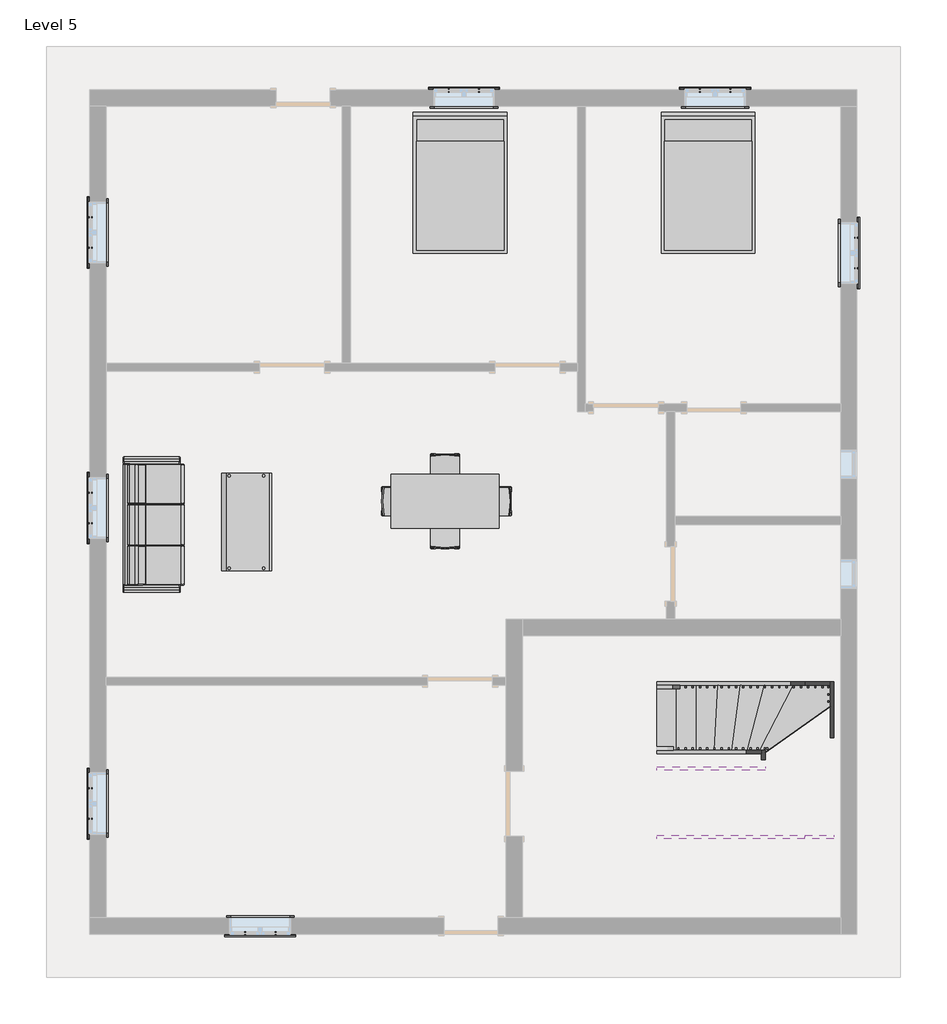
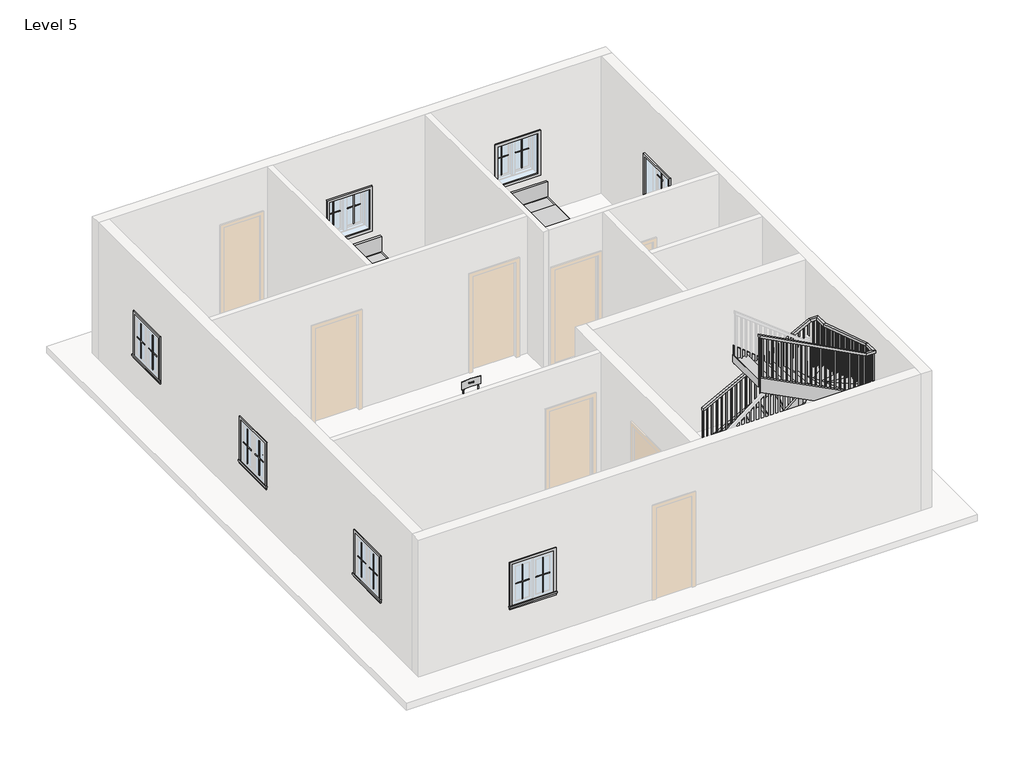
# One storey, part 2 of 2: 29 proxies, 8 members, 4 furniture elements, 1 railing, 1 stair flight.
"""IFC4 building model written with IfcOpenShell, lengths in millimetres."""

from ifc_helpers import new_model, si_unit, frame, origin, place, context, project, spatial, polyline, outline, extrude, faceted_brep, transform, mapped, element, save
from components import modern_coffee_table_17989_modern_coffee_table_17989_d3a860c8, muntin_pattern_2x2_muntin_pattern_2x2_b3fe6957, muntin_pattern_2x2_muntin_pattern_2x2_3e0ecaf2, trim_window_exterior_flat_with_sill_41619996, trim_window_interior_flat_picture_frame_51c85655, furniture_2fc85b74, furniture_29a9adb8, furniture_57072a26, bed_17739_bed_17739_15c61121, dining_table_w_chairs_11374_0cdfc61b, stair_flight_9e462077

model = new_model("IFC4")

# Units and contexts
model_context = context("Model", 3, world=origin())
ifc_project = project(units=[si_unit("LENGTHUNIT", "METRE", prefix="MILLI")], contexts=[model_context])

# Site, building, storey
site = spatial("IfcSite", under=ifc_project)
building = spatial("IfcBuilding", under=site)
storey = spatial("IfcBuildingStorey", under=building, Name="Level 5", Elevation=9601.2)

# Proxies
placement = place(None, origin())
modern_coffee_table_17989_modern_coffee_table_17989_shape = modern_coffee_table_17989_modern_coffee_table_17989_d3a860c8(model_context)
element("IfcBuildingElementProxy", 1, Name="Modern_Coffee_Table_17989 : Modern_Coffee_Table_17989", ObjectType="Modern_Coffee_Table_17989 : Modern_Coffee_Table_17989", at=placement, inside=storey, context=model_context, shape_type="MappedRepresentation", body=[
    mapped(modern_coffee_table_17989_modern_coffee_table_17989_shape, transform((-4791.7841049, 1283.3840961, 9601.2), x_axis=(0.0, 1.0, 0.0), y_axis=(-1.0, 0.0, 0.0), z_axis=(0.0, 0.0, 1.0))),
])
muntin_pattern_2x2_muntin_pattern_2x2_shape = muntin_pattern_2x2_muntin_pattern_2x2_b3fe6957(model_context)
element("IfcBuildingElementProxy", 2, Name="Muntin Pattern_2x2 : Muntin Pattern_2x2", ObjectType="Muntin Pattern_2x2 : Muntin Pattern_2x2", at=placement, inside=storey, context=model_context, shape_type="MappedRepresentation", body=[
    mapped(muntin_pattern_2x2_muntin_pattern_2x2_shape, transform((-1586.7442864, 7129.6784997, 10585.45), x_axis=(1.0, 0.0, 0.0), y_axis=(0.0, 1.0, 0.0), z_axis=(0.0, 0.0, 1.0))),
])
element("IfcBuildingElementProxy", 3, Name="Muntin Pattern_2x2 : Muntin Pattern_2x2", ObjectType="Muntin Pattern_2x2 : Muntin Pattern_2x2", at=placement, inside=storey, context=model_context, shape_type="MappedRepresentation", body=[
    mapped(muntin_pattern_2x2_muntin_pattern_2x2_shape, transform((1952.1107136, 7129.6784997, 10585.45), x_axis=(1.0, 0.0, 0.0), y_axis=(0.0, 1.0, 0.0), z_axis=(0.0, 0.0, 1.0))),
])
element("IfcBuildingElementProxy", 4, Name="Muntin Pattern_2x2 : Muntin Pattern_2x2", ObjectType="Muntin Pattern_2x2 : Muntin Pattern_2x2", at=placement, inside=storey, context=model_context, shape_type="MappedRepresentation", body=[
    mapped(muntin_pattern_2x2_muntin_pattern_2x2_shape, transform((-6633.4067864, 4915.1159997, 10585.45), x_axis=(0.0, 1.0, 0.0), y_axis=(-1.0, 0.0, 0.0), z_axis=(0.0, 0.0, 1.0))),
])
element("IfcBuildingElementProxy", 5, Name="Muntin Pattern_2x2 : Muntin Pattern_2x2", ObjectType="Muntin Pattern_2x2 : Muntin Pattern_2x2", at=placement, inside=storey, context=model_context, shape_type="MappedRepresentation", body=[
    mapped(muntin_pattern_2x2_muntin_pattern_2x2_shape, transform((-6633.4067864, 1038.4409997, 10585.45), x_axis=(0.0, 1.0, 0.0), y_axis=(-1.0, 0.0, 0.0), z_axis=(0.0, 0.0, 1.0))),
])
element("IfcBuildingElementProxy", 6, Name="Muntin Pattern_2x2 : Muntin Pattern_2x2", ObjectType="Muntin Pattern_2x2 : Muntin Pattern_2x2", at=placement, inside=storey, context=model_context, shape_type="MappedRepresentation", body=[
    mapped(muntin_pattern_2x2_muntin_pattern_2x2_shape, transform((4152.7032136, 5057.9909997, 10585.45), x_axis=(0.0, -1.0, 0.0), y_axis=(1.0, 0.0, 0.0), z_axis=(0.0, 0.0, 1.0))),
])
element("IfcBuildingElementProxy", 7, Name="Muntin Pattern_2x2 : Muntin Pattern_2x2", ObjectType="Muntin Pattern_2x2 : Muntin Pattern_2x2", at=placement, inside=storey, context=model_context, shape_type="MappedRepresentation", body=[
    mapped(muntin_pattern_2x2_muntin_pattern_2x2_shape, transform((-6633.4067864, -3125.2540003, 10585.45), x_axis=(0.0, 1.0, 0.0), y_axis=(-1.0, 0.0, 0.0), z_axis=(0.0, 0.0, 1.0))),
])
element("IfcBuildingElementProxy", 8, Name="Muntin Pattern_2x2 : Muntin Pattern_2x2", ObjectType="Muntin Pattern_2x2 : Muntin Pattern_2x2", at=placement, inside=storey, context=model_context, shape_type="MappedRepresentation", body=[
    mapped(muntin_pattern_2x2_muntin_pattern_2x2_shape, transform((-4028.3192864, -4738.4715003, 10585.45), x_axis=(-1.0, 0.0, 0.0), y_axis=(0.0, -1.0, 0.0), z_axis=(0.0, 0.0, 1.0))),
])
muntin_pattern_2x2_muntin_pattern_2x2_2_shape = muntin_pattern_2x2_muntin_pattern_2x2_3e0ecaf2(model_context)
element("IfcBuildingElementProxy", 9, Name="Muntin Pattern_2x2 : Muntin Pattern_2x2", ObjectType="Muntin Pattern_2x2 : Muntin Pattern_2x2", at=placement, inside=storey, context=model_context, shape_type="MappedRepresentation", body=[
    mapped(muntin_pattern_2x2_muntin_pattern_2x2_2_shape, transform((-1158.1192864, 7129.6784997, 10585.45), x_axis=(-1.0, 0.0, 0.0), y_axis=(0.0, -1.0, 0.0), z_axis=(0.0, 0.0, 1.0))),
])
element("IfcBuildingElementProxy", 10, Name="Muntin Pattern_2x2 : Muntin Pattern_2x2", ObjectType="Muntin Pattern_2x2 : Muntin Pattern_2x2", at=placement, inside=storey, context=model_context, shape_type="MappedRepresentation", body=[
    mapped(muntin_pattern_2x2_muntin_pattern_2x2_2_shape, transform((2380.7357136, 7129.6784997, 10585.45), x_axis=(-1.0, 0.0, 0.0), y_axis=(0.0, -1.0, 0.0), z_axis=(0.0, 0.0, 1.0))),
])
element("IfcBuildingElementProxy", 11, Name="Muntin Pattern_2x2 : Muntin Pattern_2x2", ObjectType="Muntin Pattern_2x2 : Muntin Pattern_2x2", at=placement, inside=storey, context=model_context, shape_type="MappedRepresentation", body=[
    mapped(muntin_pattern_2x2_muntin_pattern_2x2_2_shape, transform((-6633.4067864, 5343.7409997, 10585.45), x_axis=(0.0, -1.0, 0.0), y_axis=(1.0, 0.0, 0.0), z_axis=(0.0, 0.0, 1.0))),
])
element("IfcBuildingElementProxy", 12, Name="Muntin Pattern_2x2 : Muntin Pattern_2x2", ObjectType="Muntin Pattern_2x2 : Muntin Pattern_2x2", at=placement, inside=storey, context=model_context, shape_type="MappedRepresentation", body=[
    mapped(muntin_pattern_2x2_muntin_pattern_2x2_2_shape, transform((-6633.4067864, 1467.0659997, 10585.45), x_axis=(0.0, -1.0, 0.0), y_axis=(1.0, 0.0, 0.0), z_axis=(0.0, 0.0, 1.0))),
])
element("IfcBuildingElementProxy", 13, Name="Muntin Pattern_2x2 : Muntin Pattern_2x2", ObjectType="Muntin Pattern_2x2 : Muntin Pattern_2x2", at=placement, inside=storey, context=model_context, shape_type="MappedRepresentation", body=[
    mapped(muntin_pattern_2x2_muntin_pattern_2x2_2_shape, transform((4152.7032136, 4629.3659997, 10585.45), x_axis=(0.0, 1.0, 0.0), y_axis=(-1.0, 0.0, 0.0), z_axis=(0.0, 0.0, 1.0))),
])
element("IfcBuildingElementProxy", 14, Name="Muntin Pattern_2x2 : Muntin Pattern_2x2", ObjectType="Muntin Pattern_2x2 : Muntin Pattern_2x2", at=placement, inside=storey, context=model_context, shape_type="MappedRepresentation", body=[
    mapped(muntin_pattern_2x2_muntin_pattern_2x2_2_shape, transform((-6633.4067864, -2696.6290003, 10585.45), x_axis=(0.0, -1.0, 0.0), y_axis=(1.0, 0.0, 0.0), z_axis=(0.0, 0.0, 1.0))),
])
element("IfcBuildingElementProxy", 15, Name="Muntin Pattern_2x2 : Muntin Pattern_2x2", ObjectType="Muntin Pattern_2x2 : Muntin Pattern_2x2", at=placement, inside=storey, context=model_context, shape_type="MappedRepresentation", body=[
    mapped(muntin_pattern_2x2_muntin_pattern_2x2_2_shape, transform((-4456.9442864, -4738.4715003, 10585.45), x_axis=(1.0, 0.0, 0.0), y_axis=(0.0, 1.0, 0.0), z_axis=(0.0, 0.0, 1.0))),
])
trim_window_exterior_flat_with_sill_shape = trim_window_exterior_flat_with_sill_41619996(model_context)
element("IfcBuildingElementProxy", 16, Name="Trim-Window-Exterior-Flat : with Sill", ObjectType="Trim-Window-Exterior-Flat : with Sill", at=placement, inside=storey, context=model_context, shape_type="MappedRepresentation", body=[
    mapped(trim_window_exterior_flat_with_sill_shape, transform((-1372.4317864, 7139.2034997, 11430.0), x_axis=(-1.0, 0.0, 0.0), y_axis=(0.0, 0.0, 1.0), z_axis=(0.0, 1.0, 0.0))),
])
element("IfcBuildingElementProxy", 17, Name="Trim-Window-Exterior-Flat : with Sill", ObjectType="Trim-Window-Exterior-Flat : with Sill", at=placement, inside=storey, context=model_context, shape_type="MappedRepresentation", body=[
    mapped(trim_window_exterior_flat_with_sill_shape, transform((2166.4232136, 7139.2034997, 11430.0), x_axis=(-1.0, 0.0, 0.0), y_axis=(0.0, 0.0, 1.0), z_axis=(0.0, 1.0, 0.0))),
])
element("IfcBuildingElementProxy", 18, Name="Trim-Window-Exterior-Flat : with Sill", ObjectType="Trim-Window-Exterior-Flat : with Sill", at=placement, inside=storey, context=model_context, shape_type="MappedRepresentation", body=[
    mapped(trim_window_exterior_flat_with_sill_shape, transform((-6642.9317864, 5129.4284997, 11430.0), x_axis=(0.0, -1.0, 0.0), y_axis=(0.0, 0.0, 1.0), z_axis=(-1.0, 0.0, 0.0))),
])
element("IfcBuildingElementProxy", 19, Name="Trim-Window-Exterior-Flat : with Sill", ObjectType="Trim-Window-Exterior-Flat : with Sill", at=placement, inside=storey, context=model_context, shape_type="MappedRepresentation", body=[
    mapped(trim_window_exterior_flat_with_sill_shape, transform((-6642.9317864, 1252.7534997, 11430.0), x_axis=(0.0, -1.0, 0.0), y_axis=(0.0, 0.0, 1.0), z_axis=(-1.0, 0.0, 0.0))),
])
element("IfcBuildingElementProxy", 20, Name="Trim-Window-Exterior-Flat : with Sill", ObjectType="Trim-Window-Exterior-Flat : with Sill", at=placement, inside=storey, context=model_context, shape_type="MappedRepresentation", body=[
    mapped(trim_window_exterior_flat_with_sill_shape, transform((4162.2282136, 4843.6784997, 11430.0), x_axis=(0.0, 1.0, 0.0), y_axis=(0.0, 0.0, 1.0), z_axis=(1.0, 0.0, 0.0))),
])
element("IfcBuildingElementProxy", 21, Name="Trim-Window-Exterior-Flat : with Sill", ObjectType="Trim-Window-Exterior-Flat : with Sill", at=placement, inside=storey, context=model_context, shape_type="MappedRepresentation", body=[
    mapped(trim_window_exterior_flat_with_sill_shape, transform((-6642.9317864, -2910.9415003, 11430.0), x_axis=(0.0, -1.0, 0.0), y_axis=(0.0, 0.0, 1.0), z_axis=(-1.0, 0.0, 0.0))),
])
element("IfcBuildingElementProxy", 22, Name="Trim-Window-Exterior-Flat : with Sill", ObjectType="Trim-Window-Exterior-Flat : with Sill", at=placement, inside=storey, context=model_context, shape_type="MappedRepresentation", body=[
    mapped(trim_window_exterior_flat_with_sill_shape, transform((-4242.6317864, -4747.9965003, 11430.0), x_axis=(1.0, 0.0, 0.0), y_axis=(0.0, 0.0, 1.0), z_axis=(0.0, -1.0, 0.0))),
])
trim_window_interior_flat_picture_frame_shape = trim_window_interior_flat_picture_frame_51c85655(model_context)
element("IfcBuildingElementProxy", 23, Name="Trim-Window-Interior-Flat : Picture Frame", ObjectType="Trim-Window-Interior-Flat : Picture Frame", at=placement, inside=storey, context=model_context, shape_type="MappedRepresentation", body=[
    mapped(trim_window_interior_flat_picture_frame_shape, transform((-1372.4317864, 6910.6034997, 11430.0), x_axis=(1.0, 0.0, 0.0), y_axis=(0.0, 0.0, 1.0), z_axis=(0.0, -1.0, 0.0))),
])
element("IfcBuildingElementProxy", 24, Name="Trim-Window-Interior-Flat : Picture Frame", ObjectType="Trim-Window-Interior-Flat : Picture Frame", at=placement, inside=storey, context=model_context, shape_type="MappedRepresentation", body=[
    mapped(trim_window_interior_flat_picture_frame_shape, transform((2166.4232136, 6910.6034997, 11430.0), x_axis=(1.0, 0.0, 0.0), y_axis=(0.0, 0.0, 1.0), z_axis=(0.0, -1.0, 0.0))),
])
element("IfcBuildingElementProxy", 25, Name="Trim-Window-Interior-Flat : Picture Frame", ObjectType="Trim-Window-Interior-Flat : Picture Frame", at=placement, inside=storey, context=model_context, shape_type="MappedRepresentation", body=[
    mapped(trim_window_interior_flat_picture_frame_shape, transform((-6414.3317864, 5129.4284997, 11430.0), x_axis=(0.0, 1.0, 0.0), y_axis=(0.0, 0.0, 1.0), z_axis=(1.0, 0.0, 0.0))),
])
element("IfcBuildingElementProxy", 26, Name="Trim-Window-Interior-Flat : Picture Frame", ObjectType="Trim-Window-Interior-Flat : Picture Frame", at=placement, inside=storey, context=model_context, shape_type="MappedRepresentation", body=[
    mapped(trim_window_interior_flat_picture_frame_shape, transform((-6414.3317864, 1252.7534997, 11430.0), x_axis=(0.0, 1.0, 0.0), y_axis=(0.0, 0.0, 1.0), z_axis=(1.0, 0.0, 0.0))),
])
element("IfcBuildingElementProxy", 27, Name="Trim-Window-Interior-Flat : Picture Frame", ObjectType="Trim-Window-Interior-Flat : Picture Frame", at=placement, inside=storey, context=model_context, shape_type="MappedRepresentation", body=[
    mapped(trim_window_interior_flat_picture_frame_shape, transform((3933.6282136, 4843.6784997, 11430.0), x_axis=(0.0, -1.0, 0.0), y_axis=(0.0, 0.0, 1.0), z_axis=(-1.0, 0.0, 0.0))),
])
element("IfcBuildingElementProxy", 28, Name="Trim-Window-Interior-Flat : Picture Frame", ObjectType="Trim-Window-Interior-Flat : Picture Frame", at=placement, inside=storey, context=model_context, shape_type="MappedRepresentation", body=[
    mapped(trim_window_interior_flat_picture_frame_shape, transform((-6414.3317864, -2910.9415003, 11430.0), x_axis=(0.0, 1.0, 0.0), y_axis=(0.0, 0.0, 1.0), z_axis=(1.0, 0.0, 0.0))),
])
element("IfcBuildingElementProxy", 29, Name="Trim-Window-Interior-Flat : Picture Frame", ObjectType="Trim-Window-Interior-Flat : Picture Frame", at=placement, inside=storey, context=model_context, shape_type="MappedRepresentation", body=[
    mapped(trim_window_interior_flat_picture_frame_shape, transform((-4242.6317864, -4519.3965003, 11430.0), x_axis=(-1.0, 0.0, 0.0), y_axis=(0.0, 0.0, 1.0), z_axis=(0.0, 1.0, 0.0))),
])

# Furniture
furniture_shape = furniture_2fc85b74(model_context)
furniture_2_shape = furniture_29a9adb8(model_context)
furniture_3_shape = furniture_57072a26(model_context)
element("IfcFurniture", 30, at=placement, inside=storey, context=model_context, shape_type="MappedRepresentation", body=[
    mapped(furniture_shape, transform((-5371.0104604, 1017.8034997, 9601.2), x_axis=(0.0, 1.0, 0.0), y_axis=(-1.0, 0.0, 0.0), z_axis=(0.0, 0.0, 1.0))),
    mapped(furniture_2_shape, transform((-5371.0104604, 1017.8034997, 9601.2), x_axis=(0.0, 1.0, 0.0), y_axis=(-1.0, 0.0, 0.0), z_axis=(0.0, 0.0, 1.0))),
    mapped(furniture_3_shape, transform((-5371.0104604, 1017.8034997, 9601.2), x_axis=(0.0, 1.0, 0.0), y_axis=(-1.0, 0.0, 0.0), z_axis=(0.0, 0.0, 1.0))),
])
bed_17739_bed_17739_shape = bed_17739_bed_17739_15c61121(model_context)
element("IfcFurniture", 31, ObjectType="Bed_17739 : Bed_17739", at=placement, inside=storey, context=model_context, shape_type="MappedRepresentation", body=[
    mapped(bed_17739_bed_17739_shape, transform((-1425.7717864, 5805.7034997, 9601.2), x_axis=(1.0, 0.0, 0.0), y_axis=(0.0, 1.0, 0.0), z_axis=(0.0, 0.0, 1.0))),
])
element("IfcFurniture", 32, ObjectType="Bed_17739 : Bed_17739", at=placement, inside=storey, context=model_context, shape_type="MappedRepresentation", body=[
    mapped(bed_17739_bed_17739_shape, transform((2066.7282136, 5805.7034997, 9601.2), x_axis=(1.0, 0.0, 0.0), y_axis=(0.0, 1.0, 0.0), z_axis=(0.0, 0.0, 1.0))),
])
dining_table_w_chairs_11374_shape = dining_table_w_chairs_11374_0cdfc61b(model_context)
element("IfcFurniture", 33, ObjectType="Dining_Table_w_Chairs_11374", at=placement, inside=storey, context=model_context, shape_type="MappedRepresentation", body=[
    mapped(dining_table_w_chairs_11374_shape, transform((-1657.0397106, 1252.0888157, 9601.2), x_axis=(1.0, 0.0, 0.0), y_axis=(0.0, 1.0, 0.0), z_axis=(0.0, 0.0, 1.0))),
])

# Members
element("IfcMember", 34, ObjectType="Stringer - 2\" Width", at=placement, inside=storey, context=model_context, shape_type="SweptSolid", body=[
    extrude(outline(polyline([(9830.839954, 1342.8282136), (9601.2, 1342.8282136), (9601.2, 1562.5905312), (10563.700629, 3430.2454053), (10906.5956453, 3430.2454053), (9830.839954, 1342.8282136)])), frame((0.0, -1245.3365003, 0.0), z_axis=(0.0, 1.0, 0.0), x_axis=(0.0, 0.0, 1.0)), (0.0, 0.0, 1.0), 50.8),
])
element("IfcMember", 35, ObjectType="Stringer - 2\" Width", at=placement, inside=storey, context=model_context, shape_type="SweptSolid", body=[
    extrude(outline(polyline([(3430.2454053, -1245.3365003), (3430.2454053, -1194.5365003), (3784.9599055, -1194.5365003), (3784.9599055, -1245.3365003), (3430.2454053, -1245.3365003)])), frame((0.0, 0.0, 10563.700629), z_axis=(0.0, 0.0, 1.0), x_axis=(1.0, 0.0, 0.0)), (0.0, 0.0, 1.0), 342.8950162),
])
element("IfcMember", 36, ObjectType="Stringer - 2\" Width", at=placement, inside=storey, context=model_context, shape_type="SweptSolid", body=[
    extrude(outline(polyline([(-1194.5365003, 10890.2952212), (-1194.5365003, 10601.7956453), (-1364.0589833, 10601.7956453), (-3353.5365003, 11240.1682298), (-3353.5365003, 11571.1972697), (-3316.5563831, 11571.1972697), (-1194.5365003, 10890.2952212)])), frame((3784.9599055, 0.0, 0.0), z_axis=(1.0, 0.0, 0.0), x_axis=(0.0, 1.0, 0.0)), (0.0, 0.0, 1.0), 50.8),
])
element("IfcMember", 37, ObjectType="Stringer - 2\" Width", at=placement, inside=storey, context=model_context, shape_type="SweptSolid", body=[
    extrude(outline(polyline([(3835.7599055, -3353.5365003), (3835.7599055, -3404.3365003), (3430.2454053, -3404.3365003), (3430.2454053, -3353.5365003), (3835.7599055, -3353.5365003)])), frame((0.0, 0.0, 11251.0904473), z_axis=(0.0, 0.0, 1.0), x_axis=(1.0, 0.0, 0.0)), (0.0, 0.0, 1.0), 320.1068224),
])
element("IfcMember", 38, ObjectType="Stringer - 2\" Width", at=placement, inside=storey, context=model_context, shape_type="SweptSolid", body=[
    extrude(outline(polyline([(11251.0904473, 3430.2454053), (11571.1972697, 3430.2454053), (12646.9529609, 1342.8282136), (12326.8461385, 1342.8282136), (11251.0904473, 3430.2454053)])), frame((0.0, -3404.3365003, 0.0), z_axis=(0.0, 1.0, 0.0), x_axis=(0.0, 0.0, 1.0)), (0.0, 0.0, 1.0), 50.8),
])
element("IfcMember", 39, ObjectType="Stringer - 2\" Width", at=placement, inside=storey, context=model_context, shape_type="SweptSolid", body=[
    extrude(outline(polyline([(9777.3764461, 1342.8282136), (9601.2, 1342.8282136), (9601.2, 1609.0898582), (10588.3410923, 2819.7599055), (10981.618648, 2819.7599055), (9777.3764461, 1342.8282136)])), frame((0.0, -2210.5365003, 0.0), z_axis=(0.0, 1.0, 0.0), x_axis=(0.0, 0.0, 1.0)), (0.0, 0.0, 1.0), 50.8),
])
element("IfcMember", 40, ObjectType="Stringer - 2\" Width", at=placement, inside=storey, context=model_context, shape_type="SweptSolid", body=[
    extrude(outline(polyline([(-2159.7365003, 11174.4682978), (-2159.7365003, 10629.7617647), (-2193.9787177, 10629.7617647), (-2388.3365003, 10961.665107), (-2388.3365003, 11527.3409689), (-2366.3736178, 11527.3409689), (-2159.7365003, 11174.4682978)])), frame((2819.7599055, 0.0, 0.0), z_axis=(1.0, 0.0, 0.0), x_axis=(0.0, 1.0, 0.0)), (0.0, 0.0, 1.0), 50.8),
])
element("IfcMember", 41, ObjectType="Stringer - 2\" Width", at=placement, inside=storey, context=model_context, shape_type="SweptSolid", body=[
    extrude(outline(polyline([(11134.0634131, 2870.5599055), (11527.3409689, 2870.5599055), (12773.0038432, 1342.8282136), (12379.7262875, 1342.8282136), (11134.0634131, 2870.5599055)])), frame((0.0, -2439.1365003, 0.0), z_axis=(0.0, 1.0, 0.0), x_axis=(0.0, 0.0, 1.0)), (0.0, 0.0, 1.0), 50.8),
])

# Railing
element("IfcRailing", 42, ObjectType="Handrail - Rectangular", at=placement, inside=storey, context=model_context, shape_type="SolidModel", body=[
    faceted_brep([(1342.8282136, -1245.3365003, 10684.9333333), (1342.8282136, -1245.3365003, 10627.4742652), (1342.8282136, -1296.1365003, 10627.4742652), (1342.8282136, -1296.1365003, 10684.9333333), (3600.5532757, -1245.3365003, 11878.2239201), (3613.1523402, -1245.3365003, 11827.4239201), (3613.1523402, -1296.1365003, 11827.4239201), (3600.5532757, -1296.1365003, 11878.2239201), (3784.9599055, -1245.3365003, 11878.2239201), (3784.9599055, -1245.3365003, 11827.4239201), (3734.1599055, -1296.1365003, 11827.4239201), (3734.1599055, -1296.1365003, 11878.2239201), (3784.9599055, -1532.6483825, 11878.2239201), (3784.9599055, -1540.5989586, 11827.4239201), (3734.1599055, -1540.5989586, 11827.4239201), (3734.1599055, -1532.6483825, 11878.2239201), (3784.9599055, -3066.2246182, 12370.3094132), (3784.9599055, -3074.1751943, 12319.5094132), (3734.1599055, -3074.1751943, 12319.5094132), (3734.1599055, -3066.2246182, 12370.3094132), (3784.9599055, -3353.5365003, 12370.3094132), (3784.9599055, -3353.5365003, 12319.5094132), (3734.1599055, -3302.7365003, 12319.5094132), (3734.1599055, -3302.7365003, 12370.3094132), (3600.5532757, -3353.5365003, 12370.3094132), (3587.9542112, -3353.5365003, 12319.5094132), (3587.9542112, -3302.7365003, 12319.5094132), (3600.5532757, -3302.7365003, 12370.3094132), (1342.8282136, -3353.5365003, 13563.6), (1342.8282136, -3302.7365003, 13563.6), (1342.8282136, -3302.7365003, 13506.1409318), (1342.8282136, -3353.5365003, 13506.1409318)], [[[0, 1, 2, 3]], [[1, 0, 4, 5]], [[2, 1, 5, 6]], [[3, 2, 6, 7]], [[0, 3, 7, 4]], [[5, 4, 8, 9]], [[6, 5, 9, 10]], [[7, 6, 10, 11]], [[4, 7, 11, 8]], [[9, 8, 12, 13]], [[10, 9, 13, 14]], [[11, 10, 14, 15]], [[8, 11, 15, 12]], [[13, 12, 16, 17]], [[14, 13, 17, 18]], [[15, 14, 18, 19]], [[12, 15, 19, 16]], [[17, 16, 20, 21]], [[18, 17, 21, 22]], [[19, 18, 22, 23]], [[16, 19, 23, 20]], [[21, 20, 24, 25]], [[22, 21, 25, 26]], [[23, 22, 26, 27]], [[20, 23, 27, 24]], [[28, 29, 30, 31]], [[25, 24, 28, 31]], [[26, 25, 31, 30]], [[27, 26, 30, 29]], [[24, 27, 29, 28]]]),
    extrude(outline(polyline([(13468.9284102, 1413.2349055), (12479.8666667, 1413.2349055), (12479.8666667, 1432.2849055), (13458.8597858, 1432.2849055), (13468.9284102, 1413.2349055)])), frame((0.0, -3337.6615003, 0.0), z_axis=(0.0, 1.0, 0.0), x_axis=(0.0, 0.0, 1.0)), (0.0, 0.0, 1.0), 19.05),
    extrude(outline(polyline([(13415.22908, 1514.8349055), (12479.8666667, 1514.8349055), (12479.8666667, 1533.8849055), (13405.1604556, 1533.8849055), (13415.22908, 1514.8349055)])), frame((0.0, -3337.6615003, 0.0), z_axis=(0.0, 1.0, 0.0), x_axis=(0.0, 0.0, 1.0)), (0.0, 0.0, 1.0), 19.05),
    extrude(outline(polyline([(13361.5297498, 1616.4349055), (12310.5333333, 1616.4349055), (12310.5333333, 1635.4849055), (13351.4611254, 1635.4849055), (13361.5297498, 1616.4349055)])), frame((0.0, -3337.6615003, 0.0), z_axis=(0.0, 1.0, 0.0), x_axis=(0.0, 0.0, 1.0)), (0.0, 0.0, 1.0), 19.05),
    extrude(outline(polyline([(13307.8304196, 1718.0349055), (12310.5333333, 1718.0349055), (12310.5333333, 1737.0849055), (13297.7617952, 1737.0849055), (13307.8304196, 1718.0349055)])), frame((0.0, -3337.6615003, 0.0), z_axis=(0.0, 1.0, 0.0), x_axis=(0.0, 0.0, 1.0)), (0.0, 0.0, 1.0), 19.05),
    extrude(outline(polyline([(13254.1310894, 1819.6349055), (12310.5333333, 1819.6349055), (12310.5333333, 1838.6849055), (13244.062465, 1838.6849055), (13254.1310894, 1819.6349055)])), frame((0.0, -3337.6615003, 0.0), z_axis=(0.0, 1.0, 0.0), x_axis=(0.0, 0.0, 1.0)), (0.0, 0.0, 1.0), 19.05),
    extrude(outline(polyline([(13200.4317592, 1921.2349055), (12141.2, 1921.2349055), (12141.2, 1940.2849055), (13190.3631348, 1940.2849055), (13200.4317592, 1921.2349055)])), frame((0.0, -3337.6615003, 0.0), z_axis=(0.0, 1.0, 0.0), x_axis=(0.0, 0.0, 1.0)), (0.0, 0.0, 1.0), 19.05),
    extrude(outline(polyline([(13146.732429, 2022.8349055), (12141.2, 2022.8349055), (12141.2, 2041.8849055), (13136.6638046, 2041.8849055), (13146.732429, 2022.8349055)])), frame((0.0, -3337.6615003, 0.0), z_axis=(0.0, 1.0, 0.0), x_axis=(0.0, 0.0, 1.0)), (0.0, 0.0, 1.0), 19.05),
    extrude(outline(polyline([(13093.0330988, 2124.4349055), (12141.2, 2124.4349055), (12141.2, 2143.4849055), (13082.9644744, 2143.4849055), (13093.0330988, 2124.4349055)])), frame((0.0, -3337.6615003, 0.0), z_axis=(0.0, 1.0, 0.0), x_axis=(0.0, 0.0, 1.0)), (0.0, 0.0, 1.0), 19.05),
    extrude(outline(polyline([(13039.3337686, 2226.0349055), (11971.8666667, 2226.0349055), (11971.8666667, 2245.0849055), (13029.2651442, 2245.0849055), (13039.3337686, 2226.0349055)])), frame((0.0, -3337.6615003, 0.0), z_axis=(0.0, 1.0, 0.0), x_axis=(0.0, 0.0, 1.0)), (0.0, 0.0, 1.0), 19.05),
    extrude(outline(polyline([(12985.6344384, 2327.6349055), (11971.8666667, 2327.6349055), (11971.8666667, 2346.6849055), (12975.565814, 2346.6849055), (12985.6344384, 2327.6349055)])), frame((0.0, -3337.6615003, 0.0), z_axis=(0.0, 1.0, 0.0), x_axis=(0.0, 0.0, 1.0)), (0.0, 0.0, 1.0), 19.05),
    extrude(outline(polyline([(12931.9351082, 2429.2349055), (11971.8666667, 2429.2349055), (11971.8666667, 2448.2849055), (12921.8664838, 2448.2849055), (12931.9351082, 2429.2349055)])), frame((0.0, -3337.6615003, 0.0), z_axis=(0.0, 1.0, 0.0), x_axis=(0.0, 0.0, 1.0)), (0.0, 0.0, 1.0), 19.05),
    extrude(outline(polyline([(12878.235778, 2530.8349055), (11802.5333333, 2530.8349055), (11802.5333333, 2549.8849055), (12868.1671536, 2549.8849055), (12878.235778, 2530.8349055)])), frame((0.0, -3337.6615003, 0.0), z_axis=(0.0, 1.0, 0.0), x_axis=(0.0, 0.0, 1.0)), (0.0, 0.0, 1.0), 19.05),
    extrude(outline(polyline([(12824.5364478, 2632.4349055), (11802.5333333, 2632.4349055), (11802.5333333, 2651.4849055), (12814.4678234, 2651.4849055), (12824.5364478, 2632.4349055)])), frame((0.0, -3337.6615003, 0.0), z_axis=(0.0, 1.0, 0.0), x_axis=(0.0, 0.0, 1.0)), (0.0, 0.0, 1.0), 19.05),
    extrude(outline(polyline([(12770.8371176, 2734.0349055), (11802.5333333, 2734.0349055), (11802.5333333, 2753.0849055), (12760.7684932, 2753.0849055), (12770.8371176, 2734.0349055)])), frame((0.0, -3337.6615003, 0.0), z_axis=(0.0, 1.0, 0.0), x_axis=(0.0, 0.0, 1.0)), (0.0, 0.0, 1.0), 19.05),
    extrude(outline(polyline([(12717.1377874, 2835.6349055), (11802.5333333, 2835.6349055), (11802.5333333, 2854.6849055), (12707.069163, 2854.6849055), (12717.1377874, 2835.6349055)])), frame((0.0, -3337.6615003, 0.0), z_axis=(0.0, 1.0, 0.0), x_axis=(0.0, 0.0, 1.0)), (0.0, 0.0, 1.0), 19.05),
    extrude(outline(polyline([(12663.4384572, 2937.2349055), (11633.2, 2937.2349055), (11633.2, 2956.2849055), (12653.3698328, 2956.2849055), (12663.4384572, 2937.2349055)])), frame((0.0, -3337.6615003, 0.0), z_axis=(0.0, 1.0, 0.0), x_axis=(0.0, 0.0, 1.0)), (0.0, 0.0, 1.0), 19.05),
    extrude(outline(polyline([(12609.739127, 3038.8349055), (11633.2, 3038.8349055), (11633.2, 3057.8849055), (12599.6705026, 3057.8849055), (12609.739127, 3038.8349055)])), frame((0.0, -3337.6615003, 0.0), z_axis=(0.0, 1.0, 0.0), x_axis=(0.0, 0.0, 1.0)), (0.0, 0.0, 1.0), 19.05),
    extrude(outline(polyline([(12556.0397968, 3140.4349055), (11633.2, 3140.4349055), (11633.2, 3159.4849055), (12545.9711724, 3159.4849055), (12556.0397968, 3140.4349055)])), frame((0.0, -3337.6615003, 0.0), z_axis=(0.0, 1.0, 0.0), x_axis=(0.0, 0.0, 1.0)), (0.0, 0.0, 1.0), 19.05),
    extrude(outline(polyline([(12502.3404666, 3242.0349055), (11633.2, 3242.0349055), (11633.2, 3261.0849055), (12492.2718422, 3261.0849055), (12502.3404666, 3242.0349055)])), frame((0.0, -3337.6615003, 0.0), z_axis=(0.0, 1.0, 0.0), x_axis=(0.0, 0.0, 1.0)), (0.0, 0.0, 1.0), 19.05),
    extrude(outline(polyline([(12448.6411364, 3343.6349055), (11463.8666667, 3343.6349055), (11463.8666667, 3362.6849055), (12438.572512, 3362.6849055), (12448.6411364, 3343.6349055)])), frame((0.0, -3337.6615003, 0.0), z_axis=(0.0, 1.0, 0.0), x_axis=(0.0, 0.0, 1.0)), (0.0, 0.0, 1.0), 19.05),
    extrude(outline(polyline([(12394.9418062, 3445.2349055), (11463.8666667, 3445.2349055), (11463.8666667, 3464.2849055), (12384.8731818, 3464.2849055), (12394.9418062, 3445.2349055)])), frame((0.0, -3337.6615003, 0.0), z_axis=(0.0, 1.0, 0.0), x_axis=(0.0, 0.0, 1.0)), (0.0, 0.0, 1.0), 19.05),
    extrude(outline(polyline([(12341.242476, 3546.8349055), (11463.8666667, 3546.8349055), (11463.8666667, 3565.8849055), (12331.1738516, 3565.8849055), (12341.242476, 3546.8349055)])), frame((0.0, -3337.6615003, 0.0), z_axis=(0.0, 1.0, 0.0), x_axis=(0.0, 0.0, 1.0)), (0.0, 0.0, 1.0), 19.05),
    extrude(outline(polyline([(3667.4849055, -3337.6615003), (3648.4349055, -3337.6615003), (3648.4349055, -3318.6115003), (3667.4849055, -3318.6115003), (3667.4849055, -3337.6615003)])), frame((0.0, 0.0, 11463.8666667), z_axis=(0.0, 0.0, 1.0), x_axis=(1.0, 0.0, 0.0)), (0.0, 0.0, 1.0), 855.6427466),
    extrude(outline(polyline([(3769.0849055, -3293.2115003), (3769.0849055, -3312.2615003), (3750.0349055, -3312.2615003), (3750.0349055, -3293.2115003), (3769.0849055, -3293.2115003)])), frame((0.0, 0.0, 11463.8666667), z_axis=(0.0, 0.0, 1.0), x_axis=(1.0, 0.0, 0.0)), (0.0, 0.0, 1.0), 855.6427466),
    extrude(outline(polyline([(3769.0849055, -3191.6115003), (3769.0849055, -3210.6615003), (3750.0349055, -3210.6615003), (3750.0349055, -3191.6115003), (3769.0849055, -3191.6115003)])), frame((0.0, 0.0, 11463.8666667), z_axis=(0.0, 0.0, 1.0), x_axis=(1.0, 0.0, 0.0)), (0.0, 0.0, 1.0), 855.6427466),
    extrude(outline(polyline([(3769.0849055, -3090.0115003), (3769.0849055, -3109.0615003), (3750.0349055, -3109.0615003), (3750.0349055, -3090.0115003), (3769.0849055, -3090.0115003)])), frame((0.0, 0.0, 11463.8666667), z_axis=(0.0, 0.0, 1.0), x_axis=(1.0, 0.0, 0.0)), (0.0, 0.0, 1.0), 855.6427466),
    extrude(outline(polyline([(-2988.4115003, 12291.9900316), (-2988.4115003, 11294.5333333), (-3007.4615003, 11294.5333333), (-3007.4615003, 12298.1026907), (-2988.4115003, 12291.9900316)])), frame((3750.0349055, 0.0, 0.0), z_axis=(1.0, 0.0, 0.0), x_axis=(0.0, 1.0, 0.0)), (0.0, 0.0, 1.0), 19.05),
    extrude(outline(polyline([(-2886.8115003, 12259.3891834), (-2886.8115003, 11294.5333333), (-2905.8615003, 11294.5333333), (-2905.8615003, 12265.5018425), (-2886.8115003, 12259.3891834)])), frame((3750.0349055, 0.0, 0.0), z_axis=(1.0, 0.0, 0.0), x_axis=(0.0, 1.0, 0.0)), (0.0, 0.0, 1.0), 19.05),
    extrude(outline(polyline([(-2785.2115003, 12226.7883352), (-2785.2115003, 11294.5333333), (-2804.2615003, 11294.5333333), (-2804.2615003, 12232.9009942), (-2785.2115003, 12226.7883352)])), frame((3750.0349055, 0.0, 0.0), z_axis=(1.0, 0.0, 0.0), x_axis=(0.0, 1.0, 0.0)), (0.0, 0.0, 1.0), 19.05),
    extrude(outline(polyline([(-2683.6115003, 12194.187487), (-2683.6115003, 11294.5333333), (-2702.6615003, 11294.5333333), (-2702.6615003, 12200.300146), (-2683.6115003, 12194.187487)])), frame((3750.0349055, 0.0, 0.0), z_axis=(1.0, 0.0, 0.0), x_axis=(0.0, 1.0, 0.0)), (0.0, 0.0, 1.0), 19.05),
    extrude(outline(polyline([(-2582.0115003, 12161.5866387), (-2582.0115003, 11294.5333333), (-2601.0615003, 11294.5333333), (-2601.0615003, 12167.6992978), (-2582.0115003, 12161.5866387)])), frame((3750.0349055, 0.0, 0.0), z_axis=(1.0, 0.0, 0.0), x_axis=(0.0, 1.0, 0.0)), (0.0, 0.0, 1.0), 19.05),
    extrude(outline(polyline([(-2480.4115003, 12128.9857905), (-2480.4115003, 11125.2), (-2499.4615003, 11125.2), (-2499.4615003, 12135.0984495), (-2480.4115003, 12128.9857905)])), frame((3750.0349055, 0.0, 0.0), z_axis=(1.0, 0.0, 0.0), x_axis=(0.0, 1.0, 0.0)), (0.0, 0.0, 1.0), 19.05),
    extrude(outline(polyline([(-2378.8115003, 12096.3849423), (-2378.8115003, 11125.2), (-2397.8615003, 11125.2), (-2397.8615003, 12102.4976013), (-2378.8115003, 12096.3849423)])), frame((3750.0349055, 0.0, 0.0), z_axis=(1.0, 0.0, 0.0), x_axis=(0.0, 1.0, 0.0)), (0.0, 0.0, 1.0), 19.05),
    extrude(outline(polyline([(-2277.2115003, 12063.784094), (-2277.2115003, 11125.2), (-2296.2615003, 11125.2), (-2296.2615003, 12069.8967531), (-2277.2115003, 12063.784094)])), frame((3750.0349055, 0.0, 0.0), z_axis=(1.0, 0.0, 0.0), x_axis=(0.0, 1.0, 0.0)), (0.0, 0.0, 1.0), 19.05),
    extrude(outline(polyline([(-2175.6115003, 12031.1832458), (-2175.6115003, 11125.2), (-2194.6615003, 11125.2), (-2194.6615003, 12037.2959049), (-2175.6115003, 12031.1832458)])), frame((3750.0349055, 0.0, 0.0), z_axis=(1.0, 0.0, 0.0), x_axis=(0.0, 1.0, 0.0)), (0.0, 0.0, 1.0), 19.05),
    extrude(outline(polyline([(-2074.0115003, 11998.5823976), (-2074.0115003, 11125.2), (-2093.0615003, 11125.2), (-2093.0615003, 12004.6950566), (-2074.0115003, 11998.5823976)])), frame((3750.0349055, 0.0, 0.0), z_axis=(1.0, 0.0, 0.0), x_axis=(0.0, 1.0, 0.0)), (0.0, 0.0, 1.0), 19.05),
    extrude(outline(polyline([(-1972.4115003, 11965.9815494), (-1972.4115003, 10955.8666667), (-1991.4615003, 10955.8666667), (-1991.4615003, 11972.0942084), (-1972.4115003, 11965.9815494)])), frame((3750.0349055, 0.0, 0.0), z_axis=(1.0, 0.0, 0.0), x_axis=(0.0, 1.0, 0.0)), (0.0, 0.0, 1.0), 19.05),
    extrude(outline(polyline([(-1870.8115003, 11933.3807011), (-1870.8115003, 10955.8666667), (-1889.8615003, 10955.8666667), (-1889.8615003, 11939.4933602), (-1870.8115003, 11933.3807011)])), frame((3750.0349055, 0.0, 0.0), z_axis=(1.0, 0.0, 0.0), x_axis=(0.0, 1.0, 0.0)), (0.0, 0.0, 1.0), 19.05),
    extrude(outline(polyline([(-1769.2115003, 11900.7798529), (-1769.2115003, 10955.8666667), (-1788.2615003, 10955.8666667), (-1788.2615003, 11906.892512), (-1769.2115003, 11900.7798529)])), frame((3750.0349055, 0.0, 0.0), z_axis=(1.0, 0.0, 0.0), x_axis=(0.0, 1.0, 0.0)), (0.0, 0.0, 1.0), 19.05),
    extrude(outline(polyline([(-1667.6115003, 11868.1790047), (-1667.6115003, 10955.8666667), (-1686.6615003, 10955.8666667), (-1686.6615003, 11874.2916637), (-1667.6115003, 11868.1790047)])), frame((3750.0349055, 0.0, 0.0), z_axis=(1.0, 0.0, 0.0), x_axis=(0.0, 1.0, 0.0)), (0.0, 0.0, 1.0), 19.05),
    extrude(outline(polyline([(-1566.0115003, 11835.5781565), (-1566.0115003, 10955.8666667), (-1585.0615003, 10955.8666667), (-1585.0615003, 11841.6908155), (-1566.0115003, 11835.5781565)])), frame((3750.0349055, 0.0, 0.0), z_axis=(1.0, 0.0, 0.0), x_axis=(0.0, 1.0, 0.0)), (0.0, 0.0, 1.0), 19.05),
    extrude(outline(polyline([(3769.0849055, -1464.4115003), (3769.0849055, -1483.4615003), (3750.0349055, -1483.4615003), (3750.0349055, -1464.4115003), (3769.0849055, -1464.4115003)])), frame((0.0, 0.0, 10786.5333333), z_axis=(0.0, 0.0, 1.0), x_axis=(1.0, 0.0, 0.0)), (0.0, 0.0, 1.0), 1040.8905868),
    extrude(outline(polyline([(3769.0849055, -1362.8115003), (3769.0849055, -1381.8615003), (3750.0349055, -1381.8615003), (3750.0349055, -1362.8115003), (3769.0849055, -1362.8115003)])), frame((0.0, 0.0, 10786.5333333), z_axis=(0.0, 0.0, 1.0), x_axis=(1.0, 0.0, 0.0)), (0.0, 0.0, 1.0), 1040.8905868),
    extrude(outline(polyline([(3670.1032136, -1261.2115003), (3689.1532136, -1261.2115003), (3689.1532136, -1280.2615003), (3670.1032136, -1280.2615003), (3670.1032136, -1261.2115003)])), frame((0.0, 0.0, 10786.5333333), z_axis=(0.0, 0.0, 1.0), x_axis=(1.0, 0.0, 0.0)), (0.0, 0.0, 1.0), 1040.8905868),
    extrude(outline(polyline([(11803.8252174, 3568.5032136), (10786.5333333, 3568.5032136), (10786.5333333, 3587.5532136), (11813.8938418, 3587.5532136), (11803.8252174, 3568.5032136)])), frame((0.0, -1280.2615003, 0.0), z_axis=(0.0, 1.0, 0.0), x_axis=(0.0, 0.0, 1.0)), (0.0, 0.0, 1.0), 19.05),
    extrude(outline(polyline([(11750.1258872, 3466.9032136), (10786.5333333, 3466.9032136), (10786.5333333, 3485.9532136), (11760.1945116, 3485.9532136), (11750.1258872, 3466.9032136)])), frame((0.0, -1280.2615003, 0.0), z_axis=(0.0, 1.0, 0.0), x_axis=(0.0, 0.0, 1.0)), (0.0, 0.0, 1.0), 19.05),
    extrude(outline(polyline([(11696.426557, 3365.3032136), (10786.5333333, 3365.3032136), (10786.5333333, 3384.3532136), (11706.4951814, 3384.3532136), (11696.426557, 3365.3032136)])), frame((0.0, -1280.2615003, 0.0), z_axis=(0.0, 1.0, 0.0), x_axis=(0.0, 0.0, 1.0)), (0.0, 0.0, 1.0), 19.05),
    extrude(outline(polyline([(11642.7272268, 3263.7032136), (10786.5333333, 3263.7032136), (10786.5333333, 3282.7532136), (11652.7958512, 3282.7532136), (11642.7272268, 3263.7032136)])), frame((0.0, -1280.2615003, 0.0), z_axis=(0.0, 1.0, 0.0), x_axis=(0.0, 0.0, 1.0)), (0.0, 0.0, 1.0), 19.05),
    extrude(outline(polyline([(11589.0278966, 3162.1032136), (10617.2, 3162.1032136), (10617.2, 3181.1532136), (11599.096521, 3181.1532136), (11589.0278966, 3162.1032136)])), frame((0.0, -1280.2615003, 0.0), z_axis=(0.0, 1.0, 0.0), x_axis=(0.0, 0.0, 1.0)), (0.0, 0.0, 1.0), 19.05),
    extrude(outline(polyline([(11535.3285664, 3060.5032136), (10617.2, 3060.5032136), (10617.2, 3079.5532136), (11545.3971908, 3079.5532136), (11535.3285664, 3060.5032136)])), frame((0.0, -1280.2615003, 0.0), z_axis=(0.0, 1.0, 0.0), x_axis=(0.0, 0.0, 1.0)), (0.0, 0.0, 1.0), 19.05),
    extrude(outline(polyline([(11481.6292362, 2958.9032136), (10617.2, 2958.9032136), (10617.2, 2977.9532136), (11491.6978606, 2977.9532136), (11481.6292362, 2958.9032136)])), frame((0.0, -1280.2615003, 0.0), z_axis=(0.0, 1.0, 0.0), x_axis=(0.0, 0.0, 1.0)), (0.0, 0.0, 1.0), 19.05),
    extrude(outline(polyline([(11427.929906, 2857.3032136), (10617.2, 2857.3032136), (10617.2, 2876.3532136), (11437.9985304, 2876.3532136), (11427.929906, 2857.3032136)])), frame((0.0, -1280.2615003, 0.0), z_axis=(0.0, 1.0, 0.0), x_axis=(0.0, 0.0, 1.0)), (0.0, 0.0, 1.0), 19.05),
    extrude(outline(polyline([(11374.2305758, 2755.7032136), (10447.8666667, 2755.7032136), (10447.8666667, 2774.7532136), (11384.2992002, 2774.7532136), (11374.2305758, 2755.7032136)])), frame((0.0, -1280.2615003, 0.0), z_axis=(0.0, 1.0, 0.0), x_axis=(0.0, 0.0, 1.0)), (0.0, 0.0, 1.0), 19.05),
    extrude(outline(polyline([(11320.5312456, 2654.1032136), (10447.8666667, 2654.1032136), (10447.8666667, 2673.1532136), (11330.59987, 2673.1532136), (11320.5312456, 2654.1032136)])), frame((0.0, -1280.2615003, 0.0), z_axis=(0.0, 1.0, 0.0), x_axis=(0.0, 0.0, 1.0)), (0.0, 0.0, 1.0), 19.05),
    extrude(outline(polyline([(11266.8319154, 2552.5032136), (10447.8666667, 2552.5032136), (10447.8666667, 2571.5532136), (11276.9005398, 2571.5532136), (11266.8319154, 2552.5032136)])), frame((0.0, -1280.2615003, 0.0), z_axis=(0.0, 1.0, 0.0), x_axis=(0.0, 0.0, 1.0)), (0.0, 0.0, 1.0), 19.05),
    extrude(outline(polyline([(11213.1325852, 2450.9032136), (10278.5333333, 2450.9032136), (10278.5333333, 2469.9532136), (11223.2012096, 2469.9532136), (11213.1325852, 2450.9032136)])), frame((0.0, -1280.2615003, 0.0), z_axis=(0.0, 1.0, 0.0), x_axis=(0.0, 0.0, 1.0)), (0.0, 0.0, 1.0), 19.05),
    extrude(outline(polyline([(11159.433255, 2349.3032136), (10278.5333333, 2349.3032136), (10278.5333333, 2368.3532136), (11169.5018794, 2368.3532136), (11159.433255, 2349.3032136)])), frame((0.0, -1280.2615003, 0.0), z_axis=(0.0, 1.0, 0.0), x_axis=(0.0, 0.0, 1.0)), (0.0, 0.0, 1.0), 19.05),
    extrude(outline(polyline([(11105.7339248, 2247.7032136), (10278.5333333, 2247.7032136), (10278.5333333, 2266.7532136), (11115.8025492, 2266.7532136), (11105.7339248, 2247.7032136)])), frame((0.0, -1280.2615003, 0.0), z_axis=(0.0, 1.0, 0.0), x_axis=(0.0, 0.0, 1.0)), (0.0, 0.0, 1.0), 19.05),
    extrude(outline(polyline([(11052.0345946, 2146.1032136), (10109.2, 2146.1032136), (10109.2, 2165.1532136), (11062.103219, 2165.1532136), (11052.0345946, 2146.1032136)])), frame((0.0, -1280.2615003, 0.0), z_axis=(0.0, 1.0, 0.0), x_axis=(0.0, 0.0, 1.0)), (0.0, 0.0, 1.0), 19.05),
    extrude(outline(polyline([(10998.3352644, 2044.5032136), (10109.2, 2044.5032136), (10109.2, 2063.5532136), (11008.4038888, 2063.5532136), (10998.3352644, 2044.5032136)])), frame((0.0, -1280.2615003, 0.0), z_axis=(0.0, 1.0, 0.0), x_axis=(0.0, 0.0, 1.0)), (0.0, 0.0, 1.0), 19.05),
    extrude(outline(polyline([(10944.6359342, 1942.9032136), (10109.2, 1942.9032136), (10109.2, 1961.9532136), (10954.7045586, 1961.9532136), (10944.6359342, 1942.9032136)])), frame((0.0, -1280.2615003, 0.0), z_axis=(0.0, 1.0, 0.0), x_axis=(0.0, 0.0, 1.0)), (0.0, 0.0, 1.0), 19.05),
    extrude(outline(polyline([(10890.936604, 1841.3032136), (9939.8666667, 1841.3032136), (9939.8666667, 1860.3532136), (10901.0052284, 1860.3532136), (10890.936604, 1841.3032136)])), frame((0.0, -1280.2615003, 0.0), z_axis=(0.0, 1.0, 0.0), x_axis=(0.0, 0.0, 1.0)), (0.0, 0.0, 1.0), 19.05),
    extrude(outline(polyline([(10837.2372738, 1739.7032136), (9939.8666667, 1739.7032136), (9939.8666667, 1758.7532136), (10847.3058982, 1758.7532136), (10837.2372738, 1739.7032136)])), frame((0.0, -1280.2615003, 0.0), z_axis=(0.0, 1.0, 0.0), x_axis=(0.0, 0.0, 1.0)), (0.0, 0.0, 1.0), 19.05),
    extrude(outline(polyline([(10783.5379436, 1638.1032136), (9939.8666667, 1638.1032136), (9939.8666667, 1657.1532136), (10793.606568, 1657.1532136), (10783.5379436, 1638.1032136)])), frame((0.0, -1280.2615003, 0.0), z_axis=(0.0, 1.0, 0.0), x_axis=(0.0, 0.0, 1.0)), (0.0, 0.0, 1.0), 19.05),
    extrude(outline(polyline([(10729.8386134, 1536.5032136), (9770.5333333, 1536.5032136), (9770.5333333, 1555.5532136), (10739.9072378, 1555.5532136), (10729.8386134, 1536.5032136)])), frame((0.0, -1280.2615003, 0.0), z_axis=(0.0, 1.0, 0.0), x_axis=(0.0, 0.0, 1.0)), (0.0, 0.0, 1.0), 19.05),
    extrude(outline(polyline([(10676.1392831, 1434.9032136), (9770.5333333, 1434.9032136), (9770.5333333, 1453.9532136), (10686.2079076, 1453.9532136), (10676.1392831, 1434.9032136)])), frame((0.0, -1280.2615003, 0.0), z_axis=(0.0, 1.0, 0.0), x_axis=(0.0, 0.0, 1.0)), (0.0, 0.0, 1.0), 19.05),
    extrude(outline(polyline([(3769.0849055, -3318.6115003), (3769.0849055, -3337.6615003), (3750.0349055, -3337.6615003), (3750.0349055, -3318.6115003), (3769.0849055, -3318.6115003)])), frame((0.0, 0.0, 11463.8666667), z_axis=(0.0, 0.0, 1.0), x_axis=(1.0, 0.0, 0.0)), (0.0, 0.0, 1.0), 855.6427466),
    extrude(outline(polyline([(3750.0349055, -1261.2115003), (3769.0849055, -1261.2115003), (3769.0849055, -1280.2615003), (3750.0349055, -1280.2615003), (3750.0349055, -1261.2115003)])), frame((0.0, 0.0, 10786.5333333), z_axis=(0.0, 0.0, 1.0), x_axis=(1.0, 0.0, 0.0)), (0.0, 0.0, 1.0), 1040.8905868),
    extrude(outline(polyline([(13506.1409318, 1342.8282136), (12479.8666667, 1342.8282136), (12479.8666667, 1361.8782136), (13496.0723074, 1361.8782136), (13506.1409318, 1342.8282136)])), frame((0.0, -3337.6615003, 0.0), z_axis=(0.0, 1.0, 0.0), x_axis=(0.0, 0.0, 1.0)), (0.0, 0.0, 1.0), 19.05),
    extrude(outline(polyline([(10627.4742652, 1342.8282136), (9770.5333333, 1342.8282136), (9770.5333333, 1361.8782136), (10637.5428896, 1361.8782136), (10627.4742652, 1342.8282136)])), frame((0.0, -1280.2615003, 0.0), z_axis=(0.0, 1.0, 0.0), x_axis=(0.0, 0.0, 1.0)), (0.0, 0.0, 1.0), 19.05),
])

# Stair flight
stair_flight_shape = stair_flight_9e462077(model_context)
element("IfcStairFlight", 43, ObjectType="2\" Tread 1\" Nosing 1/4\" Riser", at=placement, inside=storey, context=model_context, shape_type="MappedRepresentation", body=[
    mapped(stair_flight_shape, transform((0.0, 0.0, 0.0), x_axis=(1.0, 0.0, 0.0), y_axis=(0.0, 1.0, 0.0), z_axis=(0.0, 0.0, 1.0))),
])

save(model, "model.ifc")

# Revit data of these elements
# Type "Modern_Coffee_Table_17989 : Modern_Coffee_Table_17989"
#   Default Elevation = 0
# Type "Muntin Pattern_2x2 : Muntin Pattern_2x2"
#   Width [instance default] = 4' - 0"
#   Thickness = 0' - 0 1/2"
#   Height [instance default] = 4' - 0"
#   Distance = 0' - 0 3/4"
#   Interior Material [instance default] = none
#   Exterior Material [instance default] = none
#   Default Elevation = 0
# Type "Trim-Window-Exterior-Flat : with Sill"
#   Trim Width = 0' - 2 1/4"
#   Trim Thickness_Picture Frame = 0' - 1 1/4"
#   Trim Thickness_with Sill = 0' - 0 3/4"
#   Sill Thickness = 0' - 1 1/4"
#   Opening Width [instance default] = 2' - 0"
#   Opening Height [instance default] = 3' - 0"
#   Default Elevation = 4' - 0"
#   Sill = yes
#   Picture Frame = no
#   Trim Material [instance default] = none
# Type "Trim-Window-Interior-Flat : Picture Frame"
#   Trim Thickness_Picture Frame = 0' - 1 1/4"
#   Trim Width = 0' - 2 1/4"
#   Trim Thickness_with Sill = 0' - 0 3/4"
#   Sill Thickness = 0' - 1 1/4"
#   Opening Width [instance default] = 2' - 0"
#   Opening Height [instance default] = 3' - 0"
#   Default Elevation = 4' - 0"
#   Sill = no
#   Picture Frame = yes
#   Trim Material [instance default] = none
# Type
#   Width [instance] = 6' - 3.19685"
#   Default Elevation = 0
# Type "Bed_17739 : Bed_17739"
#   Default Elevation = 0
# Type "Dining_Table_w_Chairs_11374"
#   Default Elevation = 0
#   Assembly Code = ""
# Type "Handrail - Rectangular"
#   Assembly Code = "C2010400"
#   built-in parameter 1008612 = 0.0416667 (stored number, unit not read)
#   built-in parameter 1008611 = 0.0416667 (stored number, unit not read)
#   built-in parameter 1008609 = 0.333333 (stored number, unit not read)
#   built-in parameter 1008604 = 0.166667 (stored number, unit not read)
#   built-in parameter 1008603 = 0.166667 (stored number, unit not read)
#   Railing Height = 3' - 0"
#   built-in parameter 1008630 = 2
#   built-in parameter 1008610 = 2
#   built-in parameter 1008618 = Baluster - Square : 3/4"
# Element 1 (IfcBuildingElementProxy, "Modern_Coffee_Table_17989 : Modern_Coffee_Table_17989")
#   Phase Created = New Construction
#   Materials on its faces: "1 Wood", "1 Glass", "1 Metal"
# Elements 2, 3, 4, 5, 6, 7, 8, 9, 10, 11, 12, 13, 14, 15 (IfcBuildingElementProxy, "Muntin Pattern_2x2 : Muntin Pattern_2x2")
#   Width = 0' - 11 5/8"
#   Height = 2' - 6 1/2"
#   Interior Material = Wood - Stained
#   Exterior Material = Clad - White
#   Phase Created = New Construction
#   Materials on its faces: "Clad - White", "Wood - Stained"
# Elements 16, 17, 18, 19, 20, 21, 22 (IfcBuildingElementProxy, "Trim-Window-Exterior-Flat : with Sill")
#   Opening Width = 2' - 10"
#   Opening Height = 3' - 0"
#   Trim Material = Clad - White
#   Phase Created = New Construction
#   Materials on its faces: "Clad - White"
# Elements 23, 24, 25, 26, 27, 28, 29 (IfcBuildingElementProxy, "Trim-Window-Interior-Flat : Picture Frame")
#   Opening Width = 2' - 10"
#   Opening Height = 3' - 0"
#   Trim Material = Wood - Stained
#   Phase Created = New Construction
#   Materials on its faces: "Wood - Stained"
# Element 30 (IfcFurniture)
#   Width = 6' - 3.19685"
#   Phase Created = New Construction
# Elements 31, 32 (IfcFurniture, "Bed_17739 : Bed_17739")
#   Phase Created = New Construction
#   Materials on its faces: "legs", "sheets", "bed frame", "Blanket"
# Element 33 (IfcFurniture, "Dining_Table_w_Chairs_11374")
#   Phase Created = New Construction
# Elements 34, 35, 36, 37, 38, 39, 40, 41 (IfcMember, "Stringer - 2\" Width")
#   Phase Created = New Construction
# Element 42 (IfcRailing, "Handrail - Rectangular")
#   Phase Created = New Construction
# Element 43 (IfcStairFlight, "2\" Tread 1\" Nosing 1/4\" Riser")
#   Phase Created = New Construction
# Materials
#   "1 Wood": class "Glass", colour RGB 81 52 39, transparency 0, Cost = 0
#   "1 Glass": class "Glass", colour RGB 236 240 239, transparency 0.85, Cost = 0
#   "1 Metal": class "Glass", colour RGB 244 244 244, transparency 0, Cost = 0
#   "Clad - White": class "Wood", colour RGB 242 242 238, transparency 0, Cost = 0
#   "Wood - Stained": class "Wood", colour RGB 224 178 126, transparency 0, Cost = 0
#   "legs": colour RGB 90 73 37, transparency 0, Cost = 0
#   "sheets": colour RGB 200 195 176, transparency 0, Cost = 0
#   "bed frame": colour RGB 90 73 37, transparency 0, Cost = 0
#   "Blanket": class "System", colour RGB 59 0 1, transparency 0, Cost = 0
